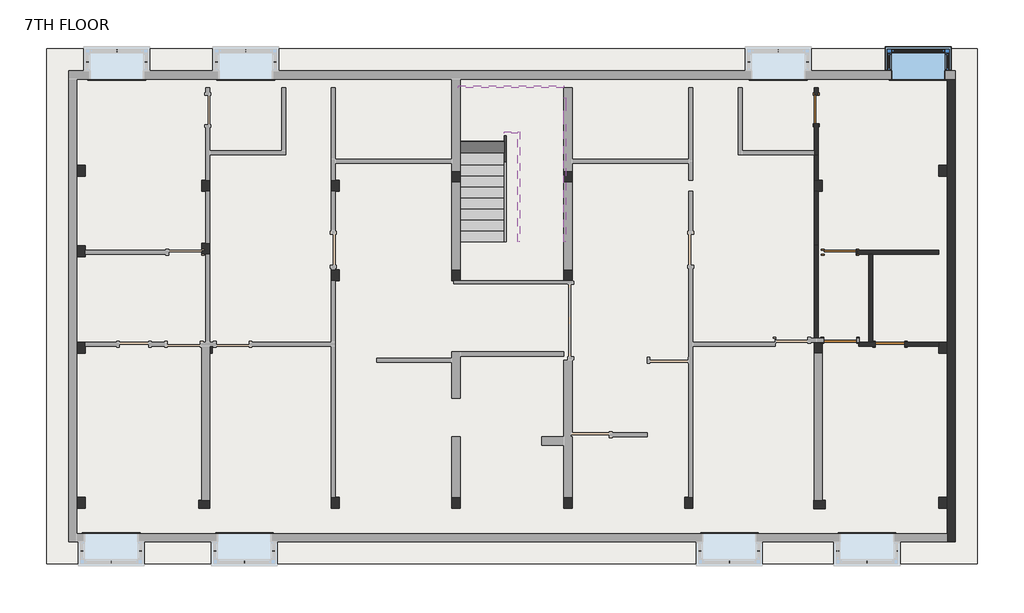
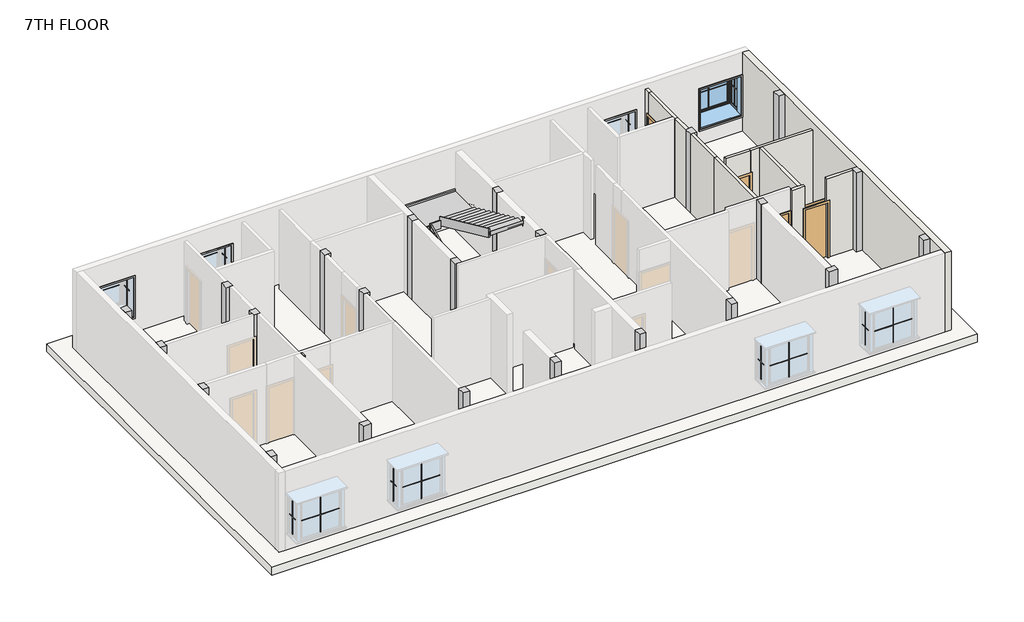
# One storey, part 2 of 2: 32 proxies, 24 columns, 11 walls, 6 members, 4 doors, 1 slab, 1 stair flight, 1 window.
"""IFC4 building model written with IfcOpenShell, lengths in millimetres."""

from ifc_helpers import new_model, si_unit, frame, origin, place, context, project, spatial, polyline, outline, extrude, faceted_brep, transform, mapped, element, save
from components import m_muntin_pattern_2x2_m_muntin_pattern_2x2_c1fd4460, m_muntin_pattern_2x2_m_muntin_pattern_2x2_777b163a, m_trim_window_interior_flat_picture_frame_44e8afef, column_f8de5b68, door_1991e9a2, door_a431d384, door_82def9da, m_door_single_panel_3_x7_f8176753, stair_flight_447a52d2, window_19bbd869

model = new_model("IFC4")

# Units and contexts
model_context = context("Model", 3, world=origin())
ifc_project = project(units=[si_unit("LENGTHUNIT", "METRE", prefix="MILLI")], contexts=[model_context])

# Site, building, storey
site = spatial("IfcSite", under=ifc_project)
building = spatial("IfcBuilding", under=site)
storey = spatial("IfcBuildingStorey", under=building, Name="7TH FLOOR", Elevation=25603.2)

# Proxies
placement = place(None, origin())
m_muntin_pattern_2x2_m_muntin_pattern_2x2_shape = m_muntin_pattern_2x2_m_muntin_pattern_2x2_c1fd4460(model_context)
element("IfcBuildingElementProxy", 1, Name="M_Muntin Pattern_2x2 : M_Muntin Pattern_2x2", ObjectType="M_Muntin Pattern_2x2 : M_Muntin Pattern_2x2", at=placement, inside=storey, context=model_context, shape_type="MappedRepresentation", body=[
    mapped(m_muntin_pattern_2x2_m_muntin_pattern_2x2_shape, transform((-11500.7987957, -5499.9182661, 26323.85), x_axis=(-1.0, 0.0, 0.0), y_axis=(0.0, -1.0, 0.0), z_axis=(0.0, 0.0, 1.0))),
])
element("IfcBuildingElementProxy", 2, Name="M_Muntin Pattern_2x2 : M_Muntin Pattern_2x2", ObjectType="M_Muntin Pattern_2x2 : M_Muntin Pattern_2x2", at=placement, inside=storey, context=model_context, shape_type="MappedRepresentation", body=[
    mapped(m_muntin_pattern_2x2_m_muntin_pattern_2x2_shape, transform((-7819.250543, -5499.9182661, 26323.85), x_axis=(-1.0, 0.0, 0.0), y_axis=(0.0, -1.0, 0.0), z_axis=(0.0, 0.0, 1.0))),
])
element("IfcBuildingElementProxy", 3, Name="M_Muntin Pattern_2x2 : M_Muntin Pattern_2x2", ObjectType="M_Muntin Pattern_2x2 : M_Muntin Pattern_2x2", at=placement, inside=storey, context=model_context, shape_type="MappedRepresentation", body=[
    mapped(m_muntin_pattern_2x2_m_muntin_pattern_2x2_shape, transform((5599.7512082, -5499.9182661, 26323.85), x_axis=(-1.0, 0.0, 0.0), y_axis=(0.0, -1.0, 0.0), z_axis=(0.0, 0.0, 1.0))),
])
element("IfcBuildingElementProxy", 4, Name="M_Muntin Pattern_2x2 : M_Muntin Pattern_2x2", ObjectType="M_Muntin Pattern_2x2 : M_Muntin Pattern_2x2", at=placement, inside=storey, context=model_context, shape_type="MappedRepresentation", body=[
    mapped(m_muntin_pattern_2x2_m_muntin_pattern_2x2_shape, transform((9408.6146942, -5499.9182662, 26323.85), x_axis=(-1.0, 0.0, 0.0), y_axis=(0.0, -1.0, 0.0), z_axis=(0.0, 0.0, 1.0))),
])
element("IfcBuildingElementProxy", 5, Name="M_Muntin Pattern_2x2 : M_Muntin Pattern_2x2", ObjectType="M_Muntin Pattern_2x2 : M_Muntin Pattern_2x2", at=placement, inside=storey, context=model_context, shape_type="MappedRepresentation", body=[
    mapped(m_muntin_pattern_2x2_m_muntin_pattern_2x2_shape, transform((-11348.3987957, 8647.7317329, 26323.85), x_axis=(1.0, 0.0, 0.0), y_axis=(0.0, 1.0, 0.0), z_axis=(0.0, 0.0, 1.0))),
])
element("IfcBuildingElementProxy", 6, Name="M_Muntin Pattern_2x2 : M_Muntin Pattern_2x2", ObjectType="M_Muntin Pattern_2x2 : M_Muntin Pattern_2x2", at=placement, inside=storey, context=model_context, shape_type="MappedRepresentation", body=[
    mapped(m_muntin_pattern_2x2_m_muntin_pattern_2x2_shape, transform((-7779.6987993, 8647.7317329, 26323.85), x_axis=(1.0, 0.0, 0.0), y_axis=(0.0, 1.0, 0.0), z_axis=(0.0, 0.0, 1.0))),
])
element("IfcBuildingElementProxy", 7, Name="M_Muntin Pattern_2x2 : M_Muntin Pattern_2x2", ObjectType="M_Muntin Pattern_2x2 : M_Muntin Pattern_2x2", at=placement, inside=storey, context=model_context, shape_type="MappedRepresentation", body=[
    mapped(m_muntin_pattern_2x2_m_muntin_pattern_2x2_shape, transform((6952.301208, 8647.7317329, 26323.85), x_axis=(1.0, 0.0, 0.0), y_axis=(0.0, 1.0, 0.0), z_axis=(0.0, 0.0, 1.0))),
])
element("IfcBuildingElementProxy", 8, Name="M_Muntin Pattern_2x2 : M_Muntin Pattern_2x2", ObjectType="M_Muntin Pattern_2x2 : M_Muntin Pattern_2x2", at=placement, inside=storey, context=model_context, shape_type="MappedRepresentation", body=[
    mapped(m_muntin_pattern_2x2_m_muntin_pattern_2x2_shape, transform((10825.8012075, 8647.7317329, 26323.85), x_axis=(1.0, 0.0, 0.0), y_axis=(0.0, 1.0, 0.0), z_axis=(0.0, 0.0, 1.0))),
])
m_muntin_pattern_2x2_m_muntin_pattern_2x2_2_shape = m_muntin_pattern_2x2_m_muntin_pattern_2x2_777b163a(model_context)
element("IfcBuildingElementProxy", 9, Name="M_Muntin Pattern_2x2 : M_Muntin Pattern_2x2", ObjectType="M_Muntin Pattern_2x2 : M_Muntin Pattern_2x2", at=placement, inside=storey, context=model_context, shape_type="MappedRepresentation", body=[
    mapped(m_muntin_pattern_2x2_m_muntin_pattern_2x2_2_shape, transform((-10690.4737957, -5190.3932661, 26323.85), x_axis=(0.0, 1.0, 0.0), y_axis=(-1.0, 0.0, 0.0), z_axis=(0.0, 0.0, 1.0))),
])
element("IfcBuildingElementProxy", 10, Name="M_Muntin Pattern_2x2 : M_Muntin Pattern_2x2", ObjectType="M_Muntin Pattern_2x2 : M_Muntin Pattern_2x2", at=placement, inside=storey, context=model_context, shape_type="MappedRepresentation", body=[
    mapped(m_muntin_pattern_2x2_m_muntin_pattern_2x2_2_shape, transform((-12311.1237957, -5190.3932661, 26323.85), x_axis=(0.0, -1.0, 0.0), y_axis=(1.0, 0.0, 0.0), z_axis=(0.0, 0.0, 1.0))),
])
element("IfcBuildingElementProxy", 11, Name="M_Muntin Pattern_2x2 : M_Muntin Pattern_2x2", ObjectType="M_Muntin Pattern_2x2 : M_Muntin Pattern_2x2", at=placement, inside=storey, context=model_context, shape_type="MappedRepresentation", body=[
    mapped(m_muntin_pattern_2x2_m_muntin_pattern_2x2_2_shape, transform((-7008.925543, -5190.3932661, 26323.85), x_axis=(0.0, 1.0, 0.0), y_axis=(-1.0, 0.0, 0.0), z_axis=(0.0, 0.0, 1.0))),
])
element("IfcBuildingElementProxy", 12, Name="M_Muntin Pattern_2x2 : M_Muntin Pattern_2x2", ObjectType="M_Muntin Pattern_2x2 : M_Muntin Pattern_2x2", at=placement, inside=storey, context=model_context, shape_type="MappedRepresentation", body=[
    mapped(m_muntin_pattern_2x2_m_muntin_pattern_2x2_2_shape, transform((-8629.575543, -5190.3932661, 26323.85), x_axis=(0.0, -1.0, 0.0), y_axis=(1.0, 0.0, 0.0), z_axis=(0.0, 0.0, 1.0))),
])
element("IfcBuildingElementProxy", 13, Name="M_Muntin Pattern_2x2 : M_Muntin Pattern_2x2", ObjectType="M_Muntin Pattern_2x2 : M_Muntin Pattern_2x2", at=placement, inside=storey, context=model_context, shape_type="MappedRepresentation", body=[
    mapped(m_muntin_pattern_2x2_m_muntin_pattern_2x2_2_shape, transform((6410.0762082, -5190.3932661, 26323.85), x_axis=(0.0, 1.0, 0.0), y_axis=(-1.0, 0.0, 0.0), z_axis=(0.0, 0.0, 1.0))),
])
element("IfcBuildingElementProxy", 14, Name="M_Muntin Pattern_2x2 : M_Muntin Pattern_2x2", ObjectType="M_Muntin Pattern_2x2 : M_Muntin Pattern_2x2", at=placement, inside=storey, context=model_context, shape_type="MappedRepresentation", body=[
    mapped(m_muntin_pattern_2x2_m_muntin_pattern_2x2_2_shape, transform((4789.4262082, -5190.3932661, 26323.85), x_axis=(0.0, -1.0, 0.0), y_axis=(1.0, 0.0, 0.0), z_axis=(0.0, 0.0, 1.0))),
])
element("IfcBuildingElementProxy", 15, Name="M_Muntin Pattern_2x2 : M_Muntin Pattern_2x2", ObjectType="M_Muntin Pattern_2x2 : M_Muntin Pattern_2x2", at=placement, inside=storey, context=model_context, shape_type="MappedRepresentation", body=[
    mapped(m_muntin_pattern_2x2_m_muntin_pattern_2x2_2_shape, transform((10218.9396942, -5190.3932662, 26323.85), x_axis=(0.0, 1.0, 0.0), y_axis=(-1.0, 0.0, 0.0), z_axis=(0.0, 0.0, 1.0))),
])
element("IfcBuildingElementProxy", 16, Name="M_Muntin Pattern_2x2 : M_Muntin Pattern_2x2", ObjectType="M_Muntin Pattern_2x2 : M_Muntin Pattern_2x2", at=placement, inside=storey, context=model_context, shape_type="MappedRepresentation", body=[
    mapped(m_muntin_pattern_2x2_m_muntin_pattern_2x2_2_shape, transform((8598.2896942, -5190.3932661, 26323.85), x_axis=(0.0, -1.0, 0.0), y_axis=(1.0, 0.0, 0.0), z_axis=(0.0, 0.0, 1.0))),
])
element("IfcBuildingElementProxy", 17, Name="M_Muntin Pattern_2x2 : M_Muntin Pattern_2x2", ObjectType="M_Muntin Pattern_2x2 : M_Muntin Pattern_2x2", at=placement, inside=storey, context=model_context, shape_type="MappedRepresentation", body=[
    mapped(m_muntin_pattern_2x2_m_muntin_pattern_2x2_2_shape, transform((-12158.7237957, 8338.2067329, 26323.85), x_axis=(0.0, -1.0, 0.0), y_axis=(1.0, 0.0, 0.0), z_axis=(0.0, 0.0, 1.0))),
])
element("IfcBuildingElementProxy", 18, Name="M_Muntin Pattern_2x2 : M_Muntin Pattern_2x2", ObjectType="M_Muntin Pattern_2x2 : M_Muntin Pattern_2x2", at=placement, inside=storey, context=model_context, shape_type="MappedRepresentation", body=[
    mapped(m_muntin_pattern_2x2_m_muntin_pattern_2x2_2_shape, transform((-10538.0737957, 8338.2067329, 26323.85), x_axis=(0.0, 1.0, 0.0), y_axis=(-1.0, 0.0, 0.0), z_axis=(0.0, 0.0, 1.0))),
])
element("IfcBuildingElementProxy", 19, Name="M_Muntin Pattern_2x2 : M_Muntin Pattern_2x2", ObjectType="M_Muntin Pattern_2x2 : M_Muntin Pattern_2x2", at=placement, inside=storey, context=model_context, shape_type="MappedRepresentation", body=[
    mapped(m_muntin_pattern_2x2_m_muntin_pattern_2x2_2_shape, transform((-8590.0237993, 8338.2067329, 26323.85), x_axis=(0.0, -1.0, 0.0), y_axis=(1.0, 0.0, 0.0), z_axis=(0.0, 0.0, 1.0))),
])
element("IfcBuildingElementProxy", 20, Name="M_Muntin Pattern_2x2 : M_Muntin Pattern_2x2", ObjectType="M_Muntin Pattern_2x2 : M_Muntin Pattern_2x2", at=placement, inside=storey, context=model_context, shape_type="MappedRepresentation", body=[
    mapped(m_muntin_pattern_2x2_m_muntin_pattern_2x2_2_shape, transform((-6969.3737993, 8338.2067329, 26323.85), x_axis=(0.0, 1.0, 0.0), y_axis=(-1.0, 0.0, 0.0), z_axis=(0.0, 0.0, 1.0))),
])
element("IfcBuildingElementProxy", 21, Name="M_Muntin Pattern_2x2 : M_Muntin Pattern_2x2", ObjectType="M_Muntin Pattern_2x2 : M_Muntin Pattern_2x2", at=placement, inside=storey, context=model_context, shape_type="MappedRepresentation", body=[
    mapped(m_muntin_pattern_2x2_m_muntin_pattern_2x2_2_shape, transform((6141.976208, 8338.2067329, 26323.85), x_axis=(0.0, -1.0, 0.0), y_axis=(1.0, 0.0, 0.0), z_axis=(0.0, 0.0, 1.0))),
])
element("IfcBuildingElementProxy", 22, Name="M_Muntin Pattern_2x2 : M_Muntin Pattern_2x2", ObjectType="M_Muntin Pattern_2x2 : M_Muntin Pattern_2x2", at=placement, inside=storey, context=model_context, shape_type="MappedRepresentation", body=[
    mapped(m_muntin_pattern_2x2_m_muntin_pattern_2x2_2_shape, transform((7762.626208, 8338.2067329, 26323.85), x_axis=(0.0, 1.0, 0.0), y_axis=(-1.0, 0.0, 0.0), z_axis=(0.0, 0.0, 1.0))),
])
element("IfcBuildingElementProxy", 23, Name="M_Muntin Pattern_2x2 : M_Muntin Pattern_2x2", ObjectType="M_Muntin Pattern_2x2 : M_Muntin Pattern_2x2", at=placement, inside=storey, context=model_context, shape_type="MappedRepresentation", body=[
    mapped(m_muntin_pattern_2x2_m_muntin_pattern_2x2_2_shape, transform((10015.4762075, 8338.2067329, 26323.85), x_axis=(0.0, -1.0, 0.0), y_axis=(1.0, 0.0, 0.0), z_axis=(0.0, 0.0, 1.0))),
])
element("IfcBuildingElementProxy", 24, Name="M_Muntin Pattern_2x2 : M_Muntin Pattern_2x2", ObjectType="M_Muntin Pattern_2x2 : M_Muntin Pattern_2x2", at=placement, inside=storey, context=model_context, shape_type="MappedRepresentation", body=[
    mapped(m_muntin_pattern_2x2_m_muntin_pattern_2x2_2_shape, transform((11636.1262075, 8338.2067329, 26323.85), x_axis=(0.0, 1.0, 0.0), y_axis=(-1.0, 0.0, 0.0), z_axis=(0.0, 0.0, 1.0))),
])
m_trim_window_interior_flat_picture_frame_shape = m_trim_window_interior_flat_picture_frame_44e8afef(model_context)
element("IfcBuildingElementProxy", 25, Name="M_Trim-Window-Interior-Flat : Picture Frame", ObjectType="M_Trim-Window-Interior-Flat : Picture Frame", at=placement, inside=storey, context=model_context, shape_type="MappedRepresentation", body=[
    mapped(m_trim_window_interior_flat_picture_frame_shape, transform((-11500.7987957, -4712.5932661, 27754.0), x_axis=(-1.0, 0.0, 0.0), y_axis=(0.0, 0.0, 1.0), z_axis=(0.0, 1.0, 0.0))),
])
element("IfcBuildingElementProxy", 26, Name="M_Trim-Window-Interior-Flat : Picture Frame", ObjectType="M_Trim-Window-Interior-Flat : Picture Frame", at=placement, inside=storey, context=model_context, shape_type="MappedRepresentation", body=[
    mapped(m_trim_window_interior_flat_picture_frame_shape, transform((-7819.250543, -4712.5932661, 27754.0), x_axis=(-1.0, 0.0, 0.0), y_axis=(0.0, 0.0, 1.0), z_axis=(0.0, 1.0, 0.0))),
])
element("IfcBuildingElementProxy", 27, Name="M_Trim-Window-Interior-Flat : Picture Frame", ObjectType="M_Trim-Window-Interior-Flat : Picture Frame", at=placement, inside=storey, context=model_context, shape_type="MappedRepresentation", body=[
    mapped(m_trim_window_interior_flat_picture_frame_shape, transform((5599.7512082, -4712.5932661, 27754.0), x_axis=(-1.0, 0.0, 0.0), y_axis=(0.0, 0.0, 1.0), z_axis=(0.0, 1.0, 0.0))),
])
element("IfcBuildingElementProxy", 28, Name="M_Trim-Window-Interior-Flat : Picture Frame", ObjectType="M_Trim-Window-Interior-Flat : Picture Frame", at=placement, inside=storey, context=model_context, shape_type="MappedRepresentation", body=[
    mapped(m_trim_window_interior_flat_picture_frame_shape, transform((9408.6146942, -4712.5932661, 27754.0), x_axis=(-1.0, 0.0, 0.0), y_axis=(0.0, 0.0, 1.0), z_axis=(0.0, 1.0, 0.0))),
])
element("IfcBuildingElementProxy", 29, Name="M_Trim-Window-Interior-Flat : Picture Frame", ObjectType="M_Trim-Window-Interior-Flat : Picture Frame", at=placement, inside=storey, context=model_context, shape_type="MappedRepresentation", body=[
    mapped(m_trim_window_interior_flat_picture_frame_shape, transform((-11348.3987957, 7860.4067329, 27754.0), x_axis=(1.0, 0.0, 0.0), y_axis=(0.0, 0.0, 1.0), z_axis=(0.0, -1.0, 0.0))),
])
element("IfcBuildingElementProxy", 30, Name="M_Trim-Window-Interior-Flat : Picture Frame", ObjectType="M_Trim-Window-Interior-Flat : Picture Frame", at=placement, inside=storey, context=model_context, shape_type="MappedRepresentation", body=[
    mapped(m_trim_window_interior_flat_picture_frame_shape, transform((-7779.6987993, 7860.4067329, 27754.0), x_axis=(1.0, 0.0, 0.0), y_axis=(0.0, 0.0, 1.0), z_axis=(0.0, -1.0, 0.0))),
])
element("IfcBuildingElementProxy", 31, Name="M_Trim-Window-Interior-Flat : Picture Frame", ObjectType="M_Trim-Window-Interior-Flat : Picture Frame", at=placement, inside=storey, context=model_context, shape_type="MappedRepresentation", body=[
    mapped(m_trim_window_interior_flat_picture_frame_shape, transform((6952.301208, 7860.4067329, 27754.0), x_axis=(1.0, 0.0, 0.0), y_axis=(0.0, 0.0, 1.0), z_axis=(0.0, -1.0, 0.0))),
])
element("IfcBuildingElementProxy", 32, Name="M_Trim-Window-Interior-Flat : Picture Frame", ObjectType="M_Trim-Window-Interior-Flat : Picture Frame", at=placement, inside=storey, context=model_context, shape_type="MappedRepresentation", body=[
    mapped(m_trim_window_interior_flat_picture_frame_shape, transform((10825.8012075, 7860.4067329, 27754.0), x_axis=(1.0, 0.0, 0.0), y_axis=(0.0, 0.0, 1.0), z_axis=(0.0, -1.0, 0.0))),
])

# Columns
element("IfcColumn", 33, ObjectType="Rectangular Column : 1'X 9\"", at=placement, inside=storey, context=model_context, shape_type="SweptSolid", body=[
    extrude(outline(polyline([(-12224.6987957, -3709.2932671), (-12224.6987957, -4014.0932671), (-12453.2987957, -4014.0932671), (-12453.2987957, -3709.2932671), (-12224.6987957, -3709.2932671)])), frame((0.0, 0.0, 25603.2), z_axis=(0.0, 0.0, 1.0), x_axis=(1.0, 0.0, 0.0)), (0.0, 0.0, 1.0), 3048.0),
])
element("IfcColumn", 34, ObjectType="Rectangular Column : 1'X 9\"", at=placement, inside=storey, context=model_context, shape_type="SweptSolid", body=[
    extrude(outline(polyline([(-12224.6987957, 583.3067334), (-12224.6987957, 278.5067334), (-12453.2987957, 278.5067334), (-12453.2987957, 583.3067334), (-12224.6987957, 583.3067334)])), frame((0.0, 0.0, 25603.2), z_axis=(0.0, 0.0, 1.0), x_axis=(1.0, 0.0, 0.0)), (0.0, 0.0, 1.0), 3048.0),
])
element("IfcColumn", 35, ObjectType="Rectangular Column : 1'X 9\"", at=placement, inside=storey, context=model_context, shape_type="SweptSolid", body=[
    extrude(outline(polyline([(-12224.6987957, 3256.6567332), (-12224.6987957, 2951.8567332), (-12453.2987957, 2951.8567332), (-12453.2987957, 3256.6567332), (-12224.6987957, 3256.6567332)])), frame((0.0, 0.0, 25603.2), z_axis=(0.0, 0.0, 1.0), x_axis=(1.0, 0.0, 0.0)), (0.0, 0.0, 1.0), 3048.0),
])
element("IfcColumn", 36, ObjectType="Rectangular Column : 1'X 9\"", at=placement, inside=storey, context=model_context, shape_type="Brep", body=[
    faceted_brep([(-8770.2987992, 5066.406733, 25603.2), (-8770.2987992, 4761.606733, 25603.2), (-8884.5987992, 4761.606733, 25603.2), (-8998.8987992, 4761.606733, 25603.2), (-8998.8987992, 5066.406733, 25603.2), (-8884.5987992, 5066.406733, 25603.2), (-8770.2987992, 5066.406733, 28651.2), (-8770.2987992, 4761.606733, 28651.2), (-8884.5987992, 4761.606733, 28651.2), (-8998.8987992, 4761.606733, 28651.2), (-8998.8987992, 5066.406733, 28651.2), (-8884.5987992, 5066.406733, 28651.2)], [[[0, 1, 2, 3, 4, 5]], [[6, 7, 1, 0]], [[7, 8, 9, 3, 2, 1]], [[9, 10, 4, 3]], [[10, 11, 6, 0, 5, 4]], [[6, 11, 10, 9, 8, 7]]]),
])
element("IfcColumn", 37, ObjectType="Rectangular Column : 1'X 9\"", at=placement, inside=storey, context=model_context, shape_type="Brep", body=[
    faceted_brep([(-8770.2987992, 3326.5067332, 25603.2), (-8770.2987992, 3021.7067332, 25603.2), (-8884.598796, 3021.7067332, 25603.2), (-8998.8987992, 3021.7067332, 25603.2), (-8998.8987992, 3326.5067332, 25603.2), (-8884.5987992, 3326.5067332, 25603.2), (-8770.2987992, 3326.5067332, 28651.2), (-8770.2987992, 3021.7067332, 28651.2), (-8884.598796, 3021.7067332, 28651.2), (-8998.8987992, 3021.7067332, 28651.2), (-8998.8987992, 3326.5067332, 28651.2), (-8884.5987992, 3326.5067332, 28651.2)], [[[0, 1, 2, 3, 4, 5]], [[6, 7, 1, 0]], [[7, 8, 9, 3, 2, 1]], [[9, 10, 4, 3]], [[10, 11, 6, 0, 5, 4]], [[6, 11, 10, 9, 8, 7]]]),
])
element("IfcColumn", 38, ObjectType="Rectangular Column : 1'X 9\"", at=placement, inside=storey, context=model_context, shape_type="SweptSolid", body=[
    extrude(outline(polyline([(-8713.148796, 278.5067334), (-8771.750543, 278.5067334), (-8771.750543, 469.0067334), (-8713.148796, 469.0067334), (-8713.148796, 278.5067334)])), frame((0.0, 0.0, 25603.2), z_axis=(0.0, 0.0, 1.0), x_axis=(1.0, 0.0, 0.0)), (0.0, 0.0, 1.0), 3048.0),
])
element("IfcColumn", 39, ObjectType="Rectangular Column : 1'X 9\"", at=placement, inside=storey, context=model_context, shape_type="Brep", body=[
    faceted_brep([(-5188.8987995, 5066.406733, 25603.2), (-5188.8987995, 4761.606733, 25603.2), (-5303.1987995, 4761.606733, 25603.2), (-5417.4987995, 4761.606733, 25603.2), (-5417.4987995, 5066.406733, 25603.2), (-5303.1987995, 5066.406733, 25603.2), (-5188.8987995, 5066.406733, 28651.2), (-5188.8987995, 4761.606733, 28651.2), (-5303.1987995, 4761.606733, 28651.2), (-5417.4987995, 4761.606733, 28651.2), (-5417.4987995, 5066.406733, 28651.2), (-5303.1987995, 5066.406733, 28651.2)], [[[0, 1, 2, 3, 4, 5]], [[6, 7, 1, 0]], [[7, 8, 9, 3, 2, 1]], [[9, 10, 4, 3]], [[10, 11, 6, 0, 5, 4]], [[6, 11, 10, 9, 8, 7]]]),
])
element("IfcColumn", 40, ObjectType="Rectangular Column : 1'X 9\"", at=placement, inside=storey, context=model_context, shape_type="Brep", body=[
    faceted_brep([(-5188.8987995, 2589.9067802, 25603.2), (-5188.8987995, 2285.1067802, 25603.2), (-5303.1987995, 2285.1067802, 25603.2), (-5417.4987995, 2285.1067802, 25603.2), (-5417.4987995, 2589.9067802, 25603.2), (-5303.1987995, 2589.9067802, 25603.2), (-5188.8987995, 2589.9067802, 28651.2), (-5188.8987995, 2285.1067802, 28651.2), (-5303.1987995, 2285.1067802, 28651.2), (-5417.4987995, 2285.1067802, 28651.2), (-5417.4987995, 2589.9067802, 28651.2), (-5303.1987995, 2589.9067802, 28651.2)], [[[0, 1, 2, 3, 4, 5]], [[6, 7, 1, 0]], [[7, 8, 9, 3, 2, 1]], [[9, 10, 4, 3]], [[10, 11, 6, 0, 5, 4]], [[6, 11, 10, 9, 8, 7]]]),
])
element("IfcColumn", 41, ObjectType="Rectangular Column : 1'X 9\"", at=placement, inside=storey, context=model_context, shape_type="Brep", body=[
    faceted_brep([(-5188.8987963, -3709.2932193, 25603.2), (-5188.8987963, -4014.0932193, 25603.2), (-5417.4987963, -4014.0932193, 25603.2), (-5417.4987963, -3709.2932193, 25603.2), (-5303.1987995, -3709.2932193, 25603.2), (-5188.8987963, -3709.2932193, 28651.2), (-5188.8987963, -4014.0932193, 28651.2), (-5417.4987963, -4014.0932193, 28651.2), (-5417.4987963, -3709.2932193, 28651.2), (-5303.1987995, -3709.2932193, 28651.2)], [[[0, 1, 2, 3, 4]], [[5, 6, 1, 0]], [[6, 7, 2, 1]], [[7, 8, 3, 2]], [[8, 9, 5, 0, 4, 3]], [[5, 9, 8, 7, 6]]]),
])
element("IfcColumn", 42, ObjectType="Rectangular Column : 1'X 9\"", at=placement, inside=storey, context=model_context, shape_type="SweptSolid", body=[
    extrude(outline(polyline([(1250.0012085, -3709.2932193), (1250.0012085, -4014.0932193), (1021.4012085, -4014.0932193), (1021.4012085, -3709.2932193), (1250.0012085, -3709.2932193)])), frame((0.0, 0.0, 25603.2), z_axis=(0.0, 0.0, 1.0), x_axis=(1.0, 0.0, 0.0)), (0.0, 0.0, 1.0), 3048.0),
])
element("IfcColumn", 43, ObjectType="Rectangular Column : 1'X 9\"", at=placement, inside=storey, context=model_context, shape_type="Brep", body=[
    faceted_brep([(4590.1012082, -3709.2932193, 25603.2), (4590.1012082, -4014.0932193, 25603.2), (4361.5012082, -4014.0932193, 25603.2), (4361.5012082, -3709.2932193, 25603.2), (4475.8012082, -3709.2932193, 25603.2), (4590.1012082, -3709.2932193, 28651.2), (4590.1012082, -4014.0932193, 28651.2), (4361.5012082, -4014.0932193, 28651.2), (4361.5012082, -3709.2932193, 28651.2), (4475.8012082, -3709.2932193, 28651.2)], [[[0, 1, 2, 3, 4]], [[5, 6, 1, 0]], [[6, 7, 2, 1]], [[7, 8, 3, 2]], [[8, 9, 5, 0, 4, 3]], [[5, 9, 8, 7, 6]]]),
])
element("IfcColumn", 44, ObjectType="Rectangular Column : 1'X 9\"", at=placement, inside=storey, context=model_context, shape_type="SweptSolid", body=[
    extrude(outline(polyline([(11625.9012075, -3709.2932671), (11625.9012075, -4014.0932671), (11397.3012075, -4014.0932671), (11397.3012075, -3709.2932671), (11625.9012075, -3709.2932671)])), frame((0.0, 0.0, 25603.2), z_axis=(0.0, 0.0, 1.0), x_axis=(1.0, 0.0, 0.0)), (0.0, 0.0, 1.0), 3048.0),
])
element("IfcColumn", 45, ObjectType="Rectangular Column : 1'X 9\"", at=placement, inside=storey, context=model_context, shape_type="Brep", body=[
    faceted_brep([(11625.9012075, 583.3067295, 25603.2), (11625.9012075, 278.5067295, 25603.2), (11397.3012075, 278.5067295, 25603.2), (11397.3012075, 469.0067295, 25603.2), (11397.3012075, 583.3067295, 25603.2), (11625.9012075, 583.3067295, 28651.2), (11625.9012075, 278.5067295, 28651.2), (11397.3012075, 278.5067295, 28651.2), (11397.3012075, 469.0067295, 28651.2), (11397.3012075, 583.3067295, 28651.2)], [[[0, 1, 2, 3, 4]], [[5, 6, 1, 0]], [[6, 7, 2, 1]], [[7, 8, 9, 4, 3, 2]], [[9, 5, 0, 4]], [[5, 9, 8, 7, 6]]]),
])
element("IfcColumn", 46, ObjectType="Rectangular Column : 1'X 9\"", at=placement, inside=storey, context=model_context, shape_type="SweptSolid", body=[
    extrude(outline(polyline([(11625.9012075, 5479.1567329), (11625.9012075, 5174.3567329), (11397.3012075, 5174.3567329), (11397.3012075, 5479.1567329), (11625.9012075, 5479.1567329)])), frame((0.0, 0.0, 25603.2), z_axis=(0.0, 0.0, 1.0), x_axis=(1.0, 0.0, 0.0)), (0.0, 0.0, 1.0), 3048.0),
])
element("IfcColumn", 47, ObjectType="Rectangular Column : 1'X 9\"", at=placement, inside=storey, context=model_context, shape_type="Brep", body=[
    faceted_brep([(8172.5040565, 5065.4824989, 25603.2), (8172.5040565, 4760.6824989, 25603.2), (8057.2012047, 4760.6824989, 25603.2), (7943.9040565, 4760.6824989, 25603.2), (7943.9040565, 5065.4824989, 25603.2), (8058.2040565, 5065.4824989, 25603.2), (8172.5040565, 5065.4824989, 28651.2), (8172.5040565, 4760.6824989, 28651.2), (8057.2012047, 4760.6824989, 28651.2), (7943.9040565, 4760.6824989, 28651.2), (7943.9040565, 5065.4824989, 28651.2), (8058.2040565, 5065.4824989, 28651.2)], [[[0, 1, 2, 3, 4, 5]], [[6, 7, 1, 0]], [[7, 8, 9, 3, 2, 1]], [[9, 10, 4, 3]], [[10, 11, 6, 0, 5, 4]], [[6, 11, 10, 9, 8, 7]]]),
])
element("IfcColumn", 48, ObjectType="Rectangular Column : 1'X 9\"", at=placement, inside=storey, context=model_context, shape_type="Brep", body=[
    faceted_brep([(8171.5012047, 583.3067334, 25603.2), (8171.5012047, 278.5067334, 25603.2), (7942.9012047, 278.5067334, 25603.2), (7942.9012047, 583.3067334, 25603.2), (8000.0512079, 583.3067334, 25603.2), (8171.5012047, 583.3067334, 28651.2), (8171.5012047, 278.5067334, 28651.2), (7942.9012047, 278.5067334, 28651.2), (7942.9012047, 583.3067334, 28651.2), (8000.0512079, 583.3067334, 28651.2)], [[[0, 1, 2, 3, 4]], [[5, 6, 1, 0]], [[6, 7, 2, 1]], [[7, 8, 3, 2]], [[8, 9, 5, 0, 4, 3]], [[5, 9, 8, 7, 6]]]),
])
element("IfcColumn", 49, ObjectType="Rectangular Column : 1'X 9\"", at=placement, inside=storey, context=model_context, shape_type="Brep", body=[
    faceted_brep([(-9076.550543, -3785.4932196, 25603.2), (-9000.350543, -3785.4932196, 25603.2), (-8771.750543, -3785.4932196, 25603.2), (-8771.750543, -4014.0932196, 25603.2), (-9076.550543, -4014.0932196, 25603.2), (-9076.550543, -3785.4932196, 28651.2), (-9000.350543, -3785.4932196, 28651.2), (-8771.750543, -3785.4932196, 28651.2), (-8771.750543, -4014.0932196, 28651.2), (-9076.550543, -4014.0932196, 28651.2)], [[[0, 1, 2, 3, 4]], [[5, 6, 7, 2, 1, 0]], [[7, 8, 3, 2]], [[8, 9, 4, 3]], [[9, 5, 0, 4]], [[5, 9, 8, 7, 6]]]),
])
element("IfcColumn", 50, ObjectType="Rectangular Column : 1'X 9\"", at=placement, inside=storey, context=model_context, shape_type="SweptSolid", body=[
    extrude(outline(polyline([(-12453.2987957, 5174.3567339), (-12453.2987957, 5479.1567339), (-12224.6987957, 5479.1567339), (-12224.6987957, 5174.3567339), (-12453.2987957, 5174.3567339)])), frame((0.0, 0.0, 25603.2), z_axis=(0.0, 0.0, 1.0), x_axis=(1.0, 0.0, 0.0)), (0.0, 0.0, 1.0), 3048.0),
])
element("IfcColumn", 51, ObjectType="Rectangular Column : 1'X 9\"", at=placement, inside=storey, context=model_context, shape_type="SweptSolid", body=[
    extrude(outline(polyline([(-1845.5417538, 5320.4067329), (-1845.5417538, 5015.6067329), (-2074.1417538, 5015.6067329), (-2074.1417538, 5320.4067329), (-1845.5417538, 5320.4067329)])), frame((0.0, 0.0, 25603.2), z_axis=(0.0, 0.0, 1.0), x_axis=(1.0, 0.0, 0.0)), (0.0, 0.0, 1.0), 3048.0),
])
element("IfcColumn", 52, ObjectType="Rectangular Column : 1'X 9\"", at=placement, inside=storey, context=model_context, shape_type="SweptSolid", body=[
    extrude(outline(polyline([(1250.0012085, 5320.4067329), (1250.0012085, 5015.6067329), (1021.4012085, 5015.6067329), (1021.4012085, 5320.4067329), (1250.0012085, 5320.4067329)])), frame((0.0, 0.0, 25603.2), z_axis=(0.0, 0.0, 1.0), x_axis=(1.0, 0.0, 0.0)), (0.0, 0.0, 1.0), 3048.0),
])
element("IfcColumn", 53, ObjectType="Rectangular Column : 1'X 9\"", at=placement, inside=storey, context=model_context, shape_type="Brep", body=[
    faceted_brep([(-1845.5417538, 2589.906774, 25603.2), (-1845.5417538, 2285.106774, 25603.2), (-2020.2487998, 2285.106774, 25603.2), (-2074.1417538, 2285.106774, 25603.2), (-2074.1417538, 2589.906774, 25603.2), (-1845.5417538, 2589.906774, 28651.2), (-1845.5417538, 2285.106774, 28651.2), (-2020.2487998, 2285.106774, 28651.2), (-2074.1417538, 2285.106774, 28651.2), (-2074.1417538, 2589.906774, 28651.2)], [[[0, 1, 2, 3, 4]], [[5, 6, 1, 0]], [[6, 7, 8, 3, 2, 1]], [[8, 9, 4, 3]], [[9, 5, 0, 4]], [[5, 9, 8, 7, 6]]]),
])
element("IfcColumn", 54, ObjectType="Rectangular Column : 1'X 9\"", at=placement, inside=storey, context=model_context, shape_type="Brep", body=[
    faceted_brep([(1253.2582462, 2589.9067742, 25603.2), (1253.2582462, 2285.1067742, 25603.2), (1024.6582462, 2285.1067742, 25603.2), (1024.6582462, 2589.9067742, 25603.2), (1250.0012085, 2589.9067742, 25603.2), (1253.2582462, 2589.9067742, 28651.2), (1253.2582462, 2285.1067742, 28651.2), (1024.6582462, 2285.1067742, 28651.2), (1024.6582462, 2589.9067742, 28651.2), (1250.0012085, 2589.9067742, 28651.2)], [[[0, 1, 2, 3, 4]], [[5, 6, 1, 0]], [[6, 7, 2, 1]], [[7, 8, 3, 2]], [[8, 9, 5, 0, 4, 3]], [[5, 9, 8, 7, 6]]]),
])
element("IfcColumn", 55, ObjectType="Rectangular Column : 1'X 9\"", at=placement, inside=storey, context=model_context, shape_type="SweptSolid", body=[
    extrude(outline(polyline([(-1848.7987998, -3709.2932663), (-1848.7987998, -4014.0932663), (-2077.3987998, -4014.0932663), (-2077.3987998, -3709.2932663), (-1848.7987998, -3709.2932663)])), frame((0.0, 0.0, 25603.2), z_axis=(0.0, 0.0, 1.0), x_axis=(1.0, 0.0, 0.0)), (0.0, 0.0, 1.0), 3048.0),
])
column_shape = column_f8de5b68(model_context)
element("IfcColumn", 56, ObjectType="Rectangular Column : 1'X 9\"", at=placement, inside=storey, context=model_context, shape_type="MappedRepresentation", body=[
    mapped(column_shape, transform((8094.1646942, -3901.6914801, 0.0), x_axis=(0.0, 1.0, 0.0), y_axis=(-1.0, 0.0, 0.0), z_axis=(0.0, 0.0, 1.0))),
])

# Doors
door_shape = door_1991e9a2(model_context)
element("IfcDoor", 57, ObjectType="M_Door-Single-Panel : 2'11\"X7' 3", at=placement, inside=storey, context=model_context, shape_type="MappedRepresentation", body=[
    mapped(door_shape, transform((8664.274939, 3078.8567332, 25603.2), x_axis=(-1.0, 0.0, 0.0), y_axis=(0.0, -1.0, 0.0), z_axis=(0.0, 0.0, 1.0))),
])
door_2_shape = door_a431d384(model_context)
element("IfcDoor", 58, ObjectType="M_Door-Single-Panel : 2'7\"X7' 2", at=placement, inside=storey, context=model_context, shape_type="MappedRepresentation", body=[
    mapped(door_2_shape, transform((8000.0512079, 7021.3751452, 25603.2), x_axis=(0.0, 1.0, 0.0), y_axis=(-1.0, 0.0, 0.0), z_axis=(0.0, 0.0, 1.0))),
])
door_3_shape = door_82def9da(model_context)
element("IfcDoor", 59, ObjectType="M_Door-Single-Panel : 2'8\"X7'", at=placement, inside=storey, context=model_context, shape_type="MappedRepresentation", body=[
    mapped(door_3_shape, transform((10046.0486694, 526.1567295, 25603.2), x_axis=(-1.0, 0.0, 0.0), y_axis=(0.0, -1.0, 0.0), z_axis=(0.0, 0.0, 1.0))),
])
m_door_single_panel_3_x7_shape = m_door_single_panel_3_x7_f8176753(model_context)
element("IfcDoor", 60, ObjectType="M_Door-Single-Panel : 3'X7'", at=placement, inside=storey, context=model_context, shape_type="MappedRepresentation", body=[
    mapped(m_door_single_panel_3_x7_shape, transform((8666.8012079, 640.4567334, 25603.2), x_axis=(-1.0, 0.0, 0.0), y_axis=(0.0, -1.0, 0.0), z_axis=(0.0, 0.0, 1.0))),
])

# Members
element("IfcMember", 61, ObjectType="Stringer - 2\" Width", at=placement, inside=storey, context=model_context, shape_type="SweptSolid", body=[
    extrude(outline(polyline([(3364.6067329, 25603.2), (3364.6067329, 25803.0262721), (6445.4289342, 27203.4), (7182.0114168, 27203.4), (3661.5714168, 25603.2), (3364.6067329, 25603.2)])), frame((-1896.3417538, 0.0, 0.0), z_axis=(1.0, 0.0, 0.0), x_axis=(0.0, 1.0, 0.0)), (0.0, 0.0, 1.0), 50.8),
])
element("IfcMember", 62, ObjectType="Stringer - 2\" Width", at=placement, inside=storey, context=model_context, shape_type="SweptSolid", body=[
    extrude(outline(polyline([(-1896.3417538, 7631.8067329), (-1896.3417538, 7682.6067329), (1021.4012085, 7682.6067329), (1021.4012085, 7631.8067329), (-1896.3417538, 7631.8067329)])), frame((0.0, 0.0, 26898.6), z_axis=(0.0, 0.0, 1.0), x_axis=(1.0, 0.0, 0.0)), (0.0, 0.0, 1.0), 304.8),
])
element("IfcMember", 63, ObjectType="Stringer - 2\" Width", at=placement, inside=storey, context=model_context, shape_type="SweptSolid", body=[
    extrude(outline(polyline([(6618.562049, 26898.6), (3364.6067329, 28377.6705982), (3364.6067329, 28712.4808176), (7355.1445316, 26898.6), (6618.562049, 26898.6)])), frame((1021.4012085, 0.0, 0.0), z_axis=(1.0, 0.0, 0.0), x_axis=(0.0, 1.0, 0.0)), (0.0, 0.0, 1.0), 50.8),
])
element("IfcMember", 64, ObjectType="Stringer - 2\" Width", at=placement, inside=storey, context=model_context, shape_type="SweptSolid", body=[
    extrude(outline(polyline([(3364.6067329, 25603.2), (3364.6067329, 25803.0262721), (6361.8067329, 27165.3899085), (6361.8067329, 26830.5796892), (3661.5714168, 25603.2), (3364.6067329, 25603.2)])), frame((-629.5987998, 0.0, 0.0), z_axis=(1.0, 0.0, 0.0), x_axis=(0.0, 1.0, 0.0)), (0.0, 0.0, 1.0), 50.8),
])
element("IfcMember", 65, ObjectType="Stringer - 2\" Width", at=placement, inside=storey, context=model_context, shape_type="SweptSolid", body=[
    extrude(outline(polyline([(-629.5987998, 6361.8067329), (-629.5987998, 6412.6067329), (-248.5987915, 6412.6067329), (-248.5987915, 6361.8067329), (-629.5987998, 6361.8067329)])), frame((0.0, 0.0, 26898.6), z_axis=(0.0, 0.0, 1.0), x_axis=(1.0, 0.0, 0.0)), (0.0, 0.0, 1.0), 304.8),
])
element("IfcMember", 66, ObjectType="Stringer - 2\" Width", at=placement, inside=storey, context=model_context, shape_type="SweptSolid", body=[
    extrude(outline(polyline([(6412.6067329, 27327.0262721), (6412.6067329, 26992.2160528), (3364.6067329, 28377.6705982), (3364.6067329, 28712.4808176), (6412.6067329, 27327.0262721)])), frame((-248.5987915, 0.0, 0.0), z_axis=(1.0, 0.0, 0.0), x_axis=(0.0, 1.0, 0.0)), (0.0, 0.0, 1.0), 50.8),
])

# Slab
element("IfcSlab", 67, ObjectType="Generic - 12\"", at=placement, inside=storey, context=model_context, shape_type="SweptSolid", body=[
    extrude(outline(polyline([(12464.1012075, 8698.6067329), (12464.1012075, -5550.7932662), (-13291.4987957, -5550.7932662), (-13291.4987957, 8698.6067329), (12464.1012075, 8698.6067329)])), frame((0.0, 0.0, 25298.4), z_axis=(0.0, 0.0, 1.0), x_axis=(1.0, 0.0, 0.0)), (0.0, 0.0, 1.0), 304.8),
])

# Stair flight
stair_flight_shape = stair_flight_447a52d2(model_context)
element("IfcStairFlight", 68, ObjectType="2\" Tread 1\" Nosing 1/4\" Riser", at=placement, inside=storey, context=model_context, shape_type="MappedRepresentation", body=[
    mapped(stair_flight_shape, transform((0.0, 0.0, 0.0), x_axis=(1.0, 0.0, 0.0), y_axis=(0.0, 1.0, 0.0), z_axis=(0.0, 0.0, 1.0))),
])

# Walls
element("IfcWall", 69, ObjectType="4.5\"", at=placement, inside=storey, context=model_context, shape_type="SweptSolid", body=[
    extrude(outline(polyline([(25603.2, 9131.6486701), (28651.2, 9131.6486701), (28651.2, 8245.174939), (27736.8, 8245.174939), (27736.8, 9108.774939), (25603.2, 9108.774939), (25603.2, 9131.6486701)])), frame((0.0, 3021.7067332, 0.0), z_axis=(0.0, 1.0, 0.0), x_axis=(0.0, 0.0, 1.0)), (0.0, 0.0, 1.0), 114.3),
])
element("IfcWall", 70, ObjectType="4.5\"", at=placement, inside=storey, context=model_context, shape_type="Brep", body=[
    faceted_brep([(7942.9012079, 5764.9067329, 28651.2), (7942.9012079, 5879.2067329, 28651.2), (7942.9012079, 7415.0751452, 28651.2), (7942.9012079, 7415.0751452, 27736.8), (7942.9012079, 6627.6751452, 27736.8), (7942.9012079, 6627.6751452, 25603.2), (7942.9012079, 5879.2067329, 25603.2), (7942.9012079, 5764.9067329, 25603.2), (8057.2012079, 7415.0751452, 28651.2), (8057.2012079, 5764.9067329, 28651.2), (8057.2012079, 5764.9067329, 25603.2), (8057.2012079, 6627.6751452, 25603.2), (8057.2012079, 6627.6751452, 27736.8), (8057.2012079, 7415.0751452, 27736.8)], [[[0, 1, 2, 3, 4, 5, 6, 7]], [[8, 9, 10, 11, 12, 13]], [[10, 7, 6, 5, 11]], [[2, 1, 0, 9, 8]], [[2, 8, 13, 3]], [[12, 4, 3, 13]], [[4, 12, 11, 5]], [[0, 7, 10, 9]]]),
])
element("IfcWall", 71, ObjectType="4.5\"", at=placement, inside=storey, context=model_context, shape_type="Brep", body=[
    faceted_brep([(7942.9012079, 7631.8067329, 25603.2), (7942.9012079, 7415.0751452, 25603.2), (7942.9012079, 7415.0751452, 27736.8), (7942.9012079, 7415.0751452, 28651.2), (7942.9012079, 7631.8067329, 28651.2), (8057.2012079, 7631.8067329, 25603.2), (8057.2012079, 7631.8067329, 28651.2), (8057.2012079, 7415.0751452, 28651.2), (8057.2012079, 7415.0751452, 27736.8), (8057.2012079, 7415.0751452, 25603.2)], [[[0, 1, 2, 3, 4]], [[5, 6, 7, 8, 9]], [[1, 0, 5, 9]], [[3, 2, 1, 9, 8, 7]], [[4, 3, 7, 6]], [[0, 4, 6, 5]]]),
])
element("IfcWall", 72, ObjectType="4.5\"", at=placement, inside=storey, context=model_context, shape_type="Brep", body=[
    faceted_brep([(8057.2012047, 3270.1432417, 25603.2), (8057.2012047, 4760.6824989, 25603.2), (8057.2012047, 4760.6824989, 28651.2), (8057.2012047, 3270.1432417, 28651.2), (7942.9012047, 3270.1432417, 25603.2), (7942.9012047, 3270.1432417, 28651.2), (7942.9012047, 4760.6824989, 28651.2), (7942.9012047, 4760.6824989, 25603.2), (7943.9040565, 4760.6824989, 25603.2), (7943.9040565, 4760.6824989, 28651.2)], [[[0, 1, 2, 3]], [[4, 5, 6, 7]], [[1, 0, 4, 7, 8]], [[2, 1, 8, 7, 6, 9]], [[3, 2, 9, 6, 5]], [[0, 3, 5, 4]]]),
])
element("IfcWall", 73, ObjectType="4.5\"", at=placement, inside=storey, context=model_context, shape_type="Brep", body=[
    faceted_brep([(7942.9012079, 3270.1432417, 25603.2), (7942.9012079, 697.6067334, 25603.2), (7942.9012079, 697.6067334, 28651.2), (7942.9012079, 3270.1432417, 28651.2), (8057.2012079, 3270.1432417, 25603.2), (8057.2012079, 3270.1432417, 28651.2), (8057.2012079, 697.6067334, 28651.2), (8057.2012079, 697.6067334, 25603.2), (8000.0512079, 697.6067334, 25603.2), (8000.0512079, 697.6067334, 28651.2)], [[[0, 1, 2, 3]], [[4, 5, 6, 7]], [[1, 0, 4, 7, 8]], [[3, 2, 9, 6, 5]], [[0, 3, 5, 4]], [[2, 1, 8, 7, 6, 9]]]),
])
element("IfcWall", 74, ObjectType="4.5\"", at=placement, inside=storey, context=model_context, shape_type="SweptSolid", body=[
    extrude(outline(polyline([(8058.2040565, 5763.9824989), (8058.2040565, 5065.4824989), (7943.9040565, 5065.4824989), (7943.9040565, 5763.9824989), (8058.2040565, 5763.9824989)])), frame((0.0, 0.0, 25603.2), z_axis=(0.0, 0.0, 1.0), x_axis=(1.0, 0.0, 0.0)), (0.0, 0.0, 1.0), 3048.0),
])
element("IfcWall", 75, ObjectType="4.5\" 2", at=placement, inside=storey, context=model_context, shape_type="Brep", body=[
    faceted_brep([(9182.4486694, 469.0067295, 25603.2), (9639.6486694, 469.0067295, 25603.2), (9639.6486694, 469.0067295, 28651.2), (9182.4486694, 469.0067295, 28651.2), (9182.4486694, 583.3067295, 25603.2), (9182.4486694, 583.3067295, 28651.2), (9451.1098918, 583.3067295, 28651.2), (9565.4098918, 583.3067295, 28651.2), (9639.6486694, 583.3067295, 28651.2), (9639.6486694, 583.3067295, 25603.2), (9565.4098918, 583.3067295, 25603.2), (9451.1098918, 583.3067295, 25603.2)], [[[0, 1, 2, 3]], [[4, 5, 6, 7, 8, 9, 10, 11]], [[1, 0, 4, 11, 10, 9]], [[2, 1, 9, 8]], [[3, 2, 8, 7, 6, 5]], [[0, 3, 5, 4]]]),
])
element("IfcWall", 76, ObjectType="4.5\" 2", at=placement, inside=storey, context=model_context, shape_type="SweptSolid", body=[
    extrude(outline(polyline([(25603.2, 11397.3012075), (28651.2, 11397.3012075), (28651.2, 10443.8236977), (27736.8, 10443.8236977), (27736.8, 10452.4486694), (25603.2, 10452.4486694), (25603.2, 11397.3012075)])), frame((0.0, 469.0067295, 0.0), z_axis=(0.0, 1.0, 0.0), x_axis=(0.0, 0.0, 1.0)), (0.0, 0.0, 1.0), 114.3),
])
element("IfcWall", 77, ObjectType="4.5\" 2", at=placement, inside=storey, context=model_context, shape_type="SweptSolid", body=[
    extrude(outline(polyline([(9565.4098918, 3021.7067332), (9565.4098918, 583.3067295), (9451.1098918, 583.3067295), (9451.1098918, 3021.7067332), (9565.4098918, 3021.7067332)])), frame((0.0, 0.0, 25603.2), z_axis=(0.0, 0.0, 1.0), x_axis=(1.0, 0.0, 0.0)), (0.0, 0.0, 1.0), 3048.0),
])
element("IfcWall", 78, ObjectType="4.5\" 2", at=placement, inside=storey, context=model_context, shape_type="Brep", body=[
    faceted_brep([(9131.6486701, 3021.7067332, 25603.2), (9451.1098918, 3021.7067332, 25603.2), (9565.4098918, 3021.7067332, 25603.2), (11397.3012075, 3021.7067332, 25603.2), (11397.3012075, 3021.7067332, 28651.2), (9565.4098918, 3021.7067332, 28651.2), (9451.1098918, 3021.7067332, 28651.2), (9131.6486701, 3021.7067332, 28651.2), (9131.6486701, 3136.0067332, 25603.2), (9131.6486701, 3136.0067332, 28651.2), (11397.3012075, 3136.0067332, 28651.2), (11397.3012075, 3136.0067332, 25603.2)], [[[0, 1, 2, 3, 4, 5, 6, 7]], [[8, 9, 10, 11]], [[3, 2, 1, 0, 8, 11]], [[4, 3, 11, 10]], [[7, 6, 5, 4, 10, 9]], [[0, 7, 9, 8]]]),
])
element("IfcWall", 79, ObjectType="9\"", at=placement, inside=storey, context=model_context, shape_type="Brep", body=[
    faceted_brep([(11625.9012075, 7860.4067329, 25603.2), (11625.9012075, 5479.1567329, 25603.2), (11625.9012075, 5174.3567329, 25603.2), (11625.9012075, 583.3067295, 25603.2), (11625.9012075, 278.5067295, 25603.2), (11625.9012075, -3709.2932671, 25603.2), (11625.9012075, -4014.0932671, 25603.2), (11625.9012075, -4712.5932662, 25603.2), (11625.9012075, -4941.1932662, 25603.2), (11625.9012075, -4941.1932662, 28651.2), (11625.9012075, -4712.5932662, 28651.2), (11625.9012075, -4014.0932671, 28651.2), (11625.9012075, -3709.2932671, 28651.2), (11625.9012075, 278.5067295, 28651.2), (11625.9012075, 583.3067295, 28651.2), (11625.9012075, 5174.3567329, 28651.2), (11625.9012075, 5479.1567329, 28651.2), (11625.9012075, 7860.4067329, 28651.2), (11854.5012075, 7860.4067329, 25603.2), (11854.5012075, 7860.4067329, 28651.2), (11854.5012075, -4941.1932662, 28651.2), (11854.5012075, -4941.1932662, 25603.2)], [[[0, 1, 2, 3, 4, 5, 6, 7, 8, 9, 10, 11, 12, 13, 14, 15, 16, 17]], [[18, 19, 20, 21]], [[8, 7, 6, 5, 4, 3, 2, 1, 0, 18, 21]], [[17, 16, 15, 14, 13, 12, 11, 10, 9, 20, 19]], [[0, 17, 19, 18]], [[9, 8, 21, 20]]]),
])

# Window
window_shape = window_19bbd869(model_context)
element("IfcWindow", 80, ObjectType="4'.8\"x3'.8\"", at=placement, inside=storey, context=model_context, shape_type="MappedRepresentation", body=[
    mapped(window_shape, transform((10825.8012075, 7974.7067329, 25603.2), x_axis=(1.0, 0.0, 0.0), y_axis=(0.0, 1.0, 0.0), z_axis=(0.0, 0.0, 1.0))),
])

save(model, "model.ifc")

# Revit data of these elements
# Type "M_Muntin Pattern_2x2 : M_Muntin Pattern_2x2"
#   Width [instance default] = 3' - 11.24409"
#   Thickness = 0' - 0 1/2"
#   Height [instance default] = 3' - 11.24409"
#   Distance = 0' - 0 3/4"
#   Interior Material [instance default] = none
#   Exterior Material [instance default] = none
#   Default Elevation = 0
# Type "M_Trim-Window-Interior-Flat : Picture Frame"
#   Trim Thickness_Picture Frame = 0' - 1.1811"
#   Trim Width = 0' - 2.3622"
#   Trim Thickness_with Sill = 0' - 0.7874"
#   Sill Thickness = 0' - 1.1811"
#   Opening Width [instance default] = 1' - 11.62205"
#   Opening Height [instance default] = 2' - 11.43307"
#   Default Elevation = 3' - 11.24409"
#   Sill = no
#   Picture Frame = yes
#   Trim Material [instance default] = none
# Type "Rectangular Column : 1'X 9\""
#   Assembly Code = "B1010200"
#   Depth = 1' - 0"
#   Offset Base = 0' - 0"
#   Offset Top = 0' - 0"
#   Width = 0' - 9"
#   Material = none
# Type "M_Door-Single-Panel : 2'11\"X7' 3"
#   Type Mark = "12"
#   Construction Type Id = "DOOR"
#   Assembly Code = "C1020300"
#   Analytic Construction = "Wooden"
#   Thickness = 0' - 1.9685"
#   Thermal Resistance (R) = 2.5876 (h·ft²·°F)/BTU
#   Swing Angle [instance default] = 90.00°
#   Heat Transfer Coefficient (U) = 0.3865 BTU/(h·ft²·°F)
#   Height = 7' - 0"
#   Trim Projection Ext = 0' - 0.98425"
#   Trim Projection Int = 0' - 0.98425"
#   Trim Width = 0' - 3.14961"
#   Width = 2' - 11"
#   Define Thermal Properties by = 1
#   Panel Material = Wood - Birch - Solid Stained Light Low Gloss
#   Trim Material = Paint - Sienna
#   Visual Light Transmittance = 0
#   Solar Heat Gain Coefficient = 0
#   Function = (empty or 0)
#   Wall Closure = (empty or 0)
# Type "M_Door-Single-Panel : 2'7\"X7' 2"
#   Type Mark = "13"
#   Construction Type Id = "DOOR"
#   Assembly Code = "C1020300"
#   Analytic Construction = "Wooden"
#   Thickness = 0' - 1.9685"
#   Thermal Resistance (R) = 2.5876 (h·ft²·°F)/BTU
#   Swing Angle [instance default] = 90.00°
#   Heat Transfer Coefficient (U) = 0.3865 BTU/(h·ft²·°F)
#   Height = 7' - 0"
#   Trim Projection Ext = 0' - 0.98425"
#   Trim Projection Int = 0' - 0.98425"
#   Trim Width = 0' - 3.14961"
#   Width = 2' - 7"
#   Define Thermal Properties by = 1
#   Panel Material = Wood - Birch - Solid Stained Light Low Gloss
#   Trim Material = Paint - Sienna
#   Visual Light Transmittance = 0
#   Solar Heat Gain Coefficient = 0
#   Function = (empty or 0)
#   Wall Closure = (empty or 0)
# Type "M_Door-Single-Panel : 2'8\"X7'"
#   Type Mark = "9"
#   Construction Type Id = "DOOR"
#   Assembly Code = "C1020300"
#   Analytic Construction = "Wooden"
#   Thickness = 0' - 1.9685"
#   Thermal Resistance (R) = 2.5876 (h·ft²·°F)/BTU
#   Swing Angle [instance default] = 90.00°
#   Heat Transfer Coefficient (U) = 0.3865 BTU/(h·ft²·°F)
#   Height = 7' - 0"
#   Trim Projection Ext = 0' - 0.98425"
#   Trim Projection Int = 0' - 0.98425"
#   Trim Width = 0' - 3.14961"
#   Width = 2' - 8"
#   Define Thermal Properties by = 1
#   Panel Material = Wood - Birch - Solid Stained Light Low Gloss
#   Trim Material = Paint - Sienna
#   Visual Light Transmittance = 0
#   Solar Heat Gain Coefficient = 0
#   Function = (empty or 0)
#   Wall Closure = (empty or 0)
# Type "M_Door-Single-Panel : 3'X7'"
#   Type Mark = "11"
#   Construction Type Id = "DOOR"
#   Assembly Code = "C1020300"
#   Analytic Construction = "Wooden"
#   Thickness = 0' - 1.9685"
#   Thermal Resistance (R) = 2.5876 (h·ft²·°F)/BTU
#   Swing Angle [instance default] = 90.00°
#   Heat Transfer Coefficient (U) = 0.3865 BTU/(h·ft²·°F)
#   Height = 7' - 0"
#   Trim Projection Ext = 0' - 0.98425"
#   Trim Projection Int = 0' - 0.98425"
#   Trim Width = 0' - 3.14961"
#   Width = 3' - 0"
#   Define Thermal Properties by = 1
#   Panel Material = Wood - Birch - Solid Stained Light Low Gloss
#   Trim Material = Paint - Sienna
#   Visual Light Transmittance = 0
#   Solar Heat Gain Coefficient = 0
#   Function = (empty or 0)
#   Wall Closure = (empty or 0)
# Type "Generic - 12\""
#   Assembly Code = "B1010"
#   Function = 0
#   Layers, outside or top first: 1' - 0" no material (function 1)
# Type "4.5\""
#   Assembly Code = "B2010"
#   Layers, outside or top first: 0' - 4 1/2" no material (function 1)
# Type "4.5\" 2"
#   Assembly Code = "B2010"
#   Layers, outside or top first: 0' - 4 1/2" no material (function 1)
# Type "9\""
#   Assembly Code = "B2010"
#   Layers, outside or top first: 0' - 9" no material (function 1)
# Type "4'.8\"x3'.8\""
#   Type Mark = "20"
#   Fire Rating = "0.5h"
#   Assembly Code = "B2020100"
#   Analytic Construction = "1/8 in Pilkington single glazing"
#   Width = 4' - 11.05512"
#   Wall Thickness [instance default] = 0' - 5.90551"
#   Visual Light Transmittance = 0.9
#   Trim Width = 5' - 7.05512"
#   Trim Height = 4' - 11.05512"
#   Thermal Resistance (R) = 1.5394 (h·ft²·°F)/BTU
#   Solar Heat Gain Coefficient = 0.86
#   Rough Width = 4' - 11.64567"
#   Rough Height = 4' - 11.64567"
#   Height 1 = 5' - 1.05512"
#   Height = 4' - 11.05512"
#   Heat Transfer Coefficient (U) = 0.6496 BTU/(h·ft²·°F)
#   Depth = 1' - 11.62205"
#   Default Sill Height = 1' - 11.62205"
#   Side Muntin Visibility = yes
#   Center Muntin Visibility = yes
#   Interior Trim Visibility [instance default] = yes
#   Exterior Trim Visibility [instance default] = yes
#   Side Muntin Pattern = M_Muntin Pattern_2x2 : M_Muntin Pattern_2x2
#   Center Muntin Pattern = M_Muntin Pattern_2x2 : M_Muntin Pattern_2x2
#   Interior Trim Material = Wood - Stained
#   Exterior Trim Material = Clad - White
#   Exterior Trim = element 422966
#   Interior Trim = M_Trim-Window-Interior-Flat : Picture Frame
#   Interior Frame Material = Wood - Stained
#   Glass Panel Material = Glass
#   Exterior Frame Material = Clad - White
#   Wall Closure = (empty or 0)
# Elements 1, 2, 3, 4, 5, 6, 7, 8 (IfcBuildingElementProxy, "M_Muntin Pattern_2x2 : M_Muntin Pattern_2x2")
#   Width = 4' - 5.55512"
#   Height = 4' - 5.55512"
#   Interior Material = Wood - Stained
#   Exterior Material = Clad - White
#   Phase Created = New Construction
#   Materials on its faces: "Clad - White", "Wood - Stained"
# Elements 9, 10, 11, 12, 13, 14, 15, 16, 17, 18, 19, 20, 21, 22, 23, 24 (IfcBuildingElementProxy, "M_Muntin Pattern_2x2 : M_Muntin Pattern_2x2")
#   Width = 1' - 2.12205"
#   Height = 4' - 5.55512"
#   Interior Material = Wood - Stained
#   Exterior Material = Clad - White
#   Phase Created = New Construction
#   Materials on its faces: "Clad - White", "Wood - Stained"
# Elements 25, 26, 27, 28, 29, 30, 31, 32 (IfcBuildingElementProxy, "M_Trim-Window-Interior-Flat : Picture Frame")
#   Opening Width = 4' - 11.05512"
#   Opening Height = 5' - 1.05512"
#   Trim Material = Wood - Stained
#   Phase Created = New Construction
#   Materials on its faces: "Wood - Stained"
# Elements 33, 34, 35, 36, 37, 38, 39, 40, 41, 42, 43, 44, 45, 46, 47, 48, 49, 50, 51, 52, 53, 54, 55 (IfcColumn, "Rectangular Column : 1'X 9\"")
#   Phase Created = New Construction
#   Materials on its faces: "Default Wall"
# Element 56 (IfcColumn, "Rectangular Column : 1'X 9\"")
#   Phase Created = New Construction
# Element 57 (IfcDoor, "M_Door-Single-Panel : 2'11\"X7' 3")
#   Swing Angle = 90.00°
#   Phase Created = New Construction
#   Materials on its faces: "Paint - Sienna", "Wood - Birch - Solid Stained Light Low Gloss"
# Element 58 (IfcDoor, "M_Door-Single-Panel : 2'7\"X7' 2")
#   Swing Angle = 90.00°
#   Phase Created = New Construction
#   Materials on its faces: "Paint - Sienna", "Wood - Birch - Solid Stained Light Low Gloss"
# Element 59 (IfcDoor, "M_Door-Single-Panel : 2'8\"X7'")
#   Swing Angle = 90.00°
#   Phase Created = New Construction
#   Materials on its faces: "Paint - Sienna", "Wood - Birch - Solid Stained Light Low Gloss"
# Element 60 (IfcDoor, "M_Door-Single-Panel : 3'X7'")
#   Swing Angle = 90.00°
#   Phase Created = New Construction
#   Materials on its faces: "Paint - Sienna", "Wood - Birch - Solid Stained Light Low Gloss"
# Elements 61, 62, 63, 64, 65, 66 (IfcMember, "Stringer - 2\" Width")
#   Phase Created = New Construction
# Element 67 (IfcSlab, "Generic - 12\"")
#   Height Offset From Level = 0' - 0"
#   Phase Created = New Construction
#   Materials on its faces: "Default Floor"
# Element 68 (IfcStairFlight, "2\" Tread 1\" Nosing 1/4\" Riser")
#   Phase Created = New Construction
# Elements 69, 70, 71, 72, 73, 74 (IfcWall, "4.5\"")
#   Top Offset = -0' - 6"
#   Base Offset = 0' - 0"
#   wall height = 10' - 0"
#   Phase Created = New Construction
#   Base Constraint = 7TH FLOOR
#   Top Constraint = 8TH FLOOR
#   Materials on its faces: "Default Wall"
# Elements 75, 76, 77, 78 (IfcWall, "4.5\" 2")
#   Top Offset = -0' - 6"
#   Base Offset = 0' - 0"
#   wall height = 10' - 0"
#   Phase Created = New Construction
#   Base Constraint = 7TH FLOOR
#   Top Constraint = 8TH FLOOR
#   Materials on its faces: "Default Wall"
# Element 79 (IfcWall, "9\"")
#   Top Offset = -0' - 6"
#   Base Offset = 0' - 0"
#   wall height = 10' - 0"
#   Phase Created = New Construction
#   Base Constraint = 7TH FLOOR
#   Top Constraint = 8TH FLOOR
#   Materials on its faces: "Default Wall"
# Element 80 (IfcWindow, "4'.8\"x3'.8\"")
#   Mark = "286"
#   Interior Trim Visibility = yes
#   Exterior Trim Visibility = yes
#   Phase Created = New Construction
#   Materials on its faces: "Clad - White", "Wood - Stained", "Glass"
# Materials
#   "Wood - Birch - Solid Stained Light Low Gloss": class "Wood", colour RGB 210 159 95, transparency 0, Cost = 0
#   "Paint - Sienna": colour RGB 118 70 51, transparency 0, Cost = 0
#   "Wood - Stained": class "Wood", colour RGB 224 178 126, transparency 0, Cost = 0
#   "Clad - White": class "Wood", colour RGB 242 242 238, transparency 0, Cost = 0
#   "Glass": class "Glass", colour RGB 0 128 192, transparency 0.75, Description = "Soda Lime Glass", Cost = 0
#   "Default Wall": colour RGB 128 128 128, transparency 0, Cost = 0
#   "Default Floor": colour RGB 128 128 128, transparency 0, Cost = 0
